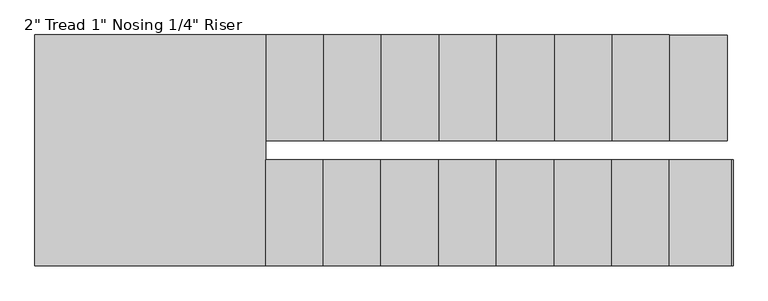
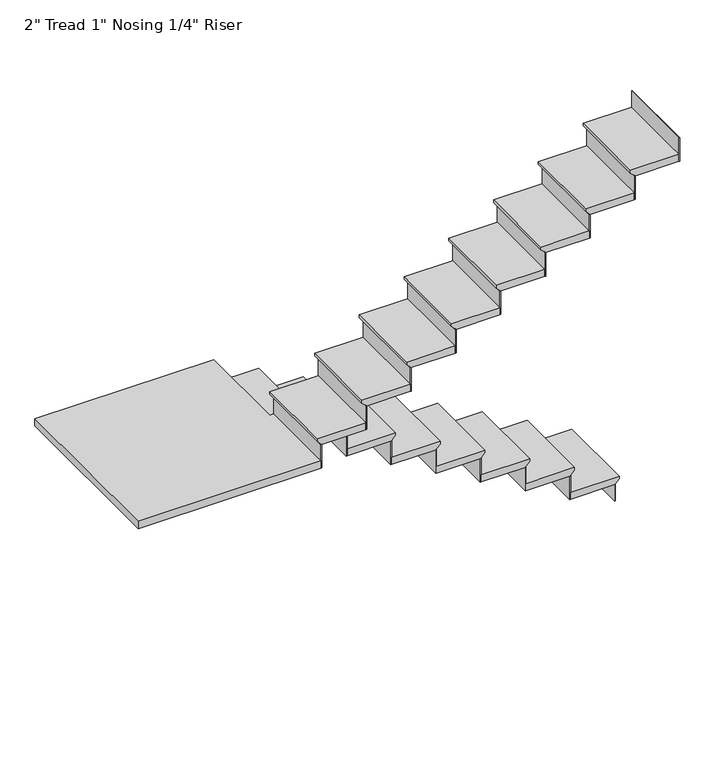
"""IFC4 building model written with IfcOpenShell, lengths in millimetres: stair flight geometry."""

from ifc_helpers import new_model, si_unit, origin, place, context, project, spatial, faceted_brep, source, transform, mapped, element, save


def stair_flight_b2054cc5(model_context):
    return source(origin(), model_context, "Body", "Brep", [
        faceted_brep([(-1805.9198569, -5306.3933037, 16152.2833333), (-1805.9198569, -5306.3933037, 16171.3333333), (-1805.9198569, -5865.1933037, 16171.3333333), (-1805.9198569, -5865.1933037, 16152.2833333), (-1831.3198569, -5306.3933037, 16126.8833333), (-1831.3198569, -5865.1933037, 16126.8833333), (-2136.1198569, -5306.3933037, 16171.3333333), (-2136.1198569, -5865.1933037, 16171.3333333), (-1831.3198569, -5865.1933037, 16120.5333333), (-2136.1198569, -5865.1933037, 16120.5333333), (-2136.1198569, -5306.3933037, 16120.5333333), (-1831.3198569, -5306.3933037, 16120.5333333)], [[[0, 1, 2, 3]], [[4, 0, 3, 5]], [[2, 1, 6, 7]], [[8, 9, 10, 11]], [[2, 7, 9, 8, 5, 3]], [[8, 11, 4, 5]], [[6, 1, 0, 4, 11, 10]], [[7, 6, 10, 9]]]),
        faceted_brep([(-1831.3198569, -5306.3933037, 16120.5333333), (-1831.3198569, -5306.3933037, 16002.0), (-1837.6698569, -5306.3933037, 16002.0), (-1837.6698569, -5306.3933037, 16120.5333333), (-1831.3198569, -5865.1933037, 16120.5333333), (-1837.6698569, -5865.1933037, 16120.5333333), (-1837.6698569, -5865.1933037, 16002.0), (-1831.3198569, -5865.1933037, 16002.0)], [[[0, 1, 2, 3]], [[4, 5, 6, 7]], [[1, 0, 4, 7]], [[2, 1, 7, 6]], [[3, 2, 6, 5]], [[0, 3, 5, 4]]]),
        faceted_brep([(-2136.1198569, -5306.3933037, 16289.8666667), (-2136.1198569, -5306.3933037, 16120.5333333), (-2142.4698569, -5306.3933037, 16120.5333333), (-2142.4698569, -5306.3933037, 16289.8666667), (-2136.1198569, -5865.1933037, 16289.8666667), (-2142.4698569, -5865.1933037, 16289.8666667), (-2142.4698569, -5865.1933037, 16120.5333333), (-2136.1198569, -5865.1933037, 16120.5333333)], [[[0, 1, 2, 3]], [[4, 5, 6, 7]], [[1, 0, 4, 7]], [[2, 1, 7, 6]], [[3, 2, 6, 5]], [[0, 3, 5, 4]]]),
        faceted_brep([(-2110.7198569, -5865.1933037, 16340.6666667), (-2110.7198569, -5306.3933037, 16340.6666667), (-2440.9198569, -5306.3933037, 16340.6666667), (-2440.9198569, -5865.1933037, 16340.6666667), (-2136.1198569, -5865.1933037, 16289.8666667), (-2440.9198569, -5865.1933037, 16289.8666667), (-2440.9198569, -5306.3933037, 16289.8666667), (-2136.1198569, -5306.3933037, 16289.8666667), (-2136.1198569, -5865.1933037, 16296.2166667), (-2110.7198569, -5865.1933037, 16321.6166667), (-2136.1198569, -5306.3933037, 16296.2166667), (-2110.7198569, -5306.3933037, 16321.6166667)], [[[0, 1, 2, 3]], [[4, 5, 6, 7]], [[0, 3, 5, 4, 8, 9]], [[4, 7, 10, 8]], [[2, 1, 11, 10, 7, 6]], [[3, 2, 6, 5]], [[11, 1, 0, 9]], [[10, 11, 9, 8]]]),
        faceted_brep([(-2440.9198569, -5306.3933037, 16459.2), (-2440.9198569, -5306.3933037, 16289.8666667), (-2447.2698569, -5306.3933037, 16289.8666667), (-2447.2698569, -5306.3933037, 16459.2), (-2440.9198569, -5865.1933037, 16459.2), (-2447.2698569, -5865.1933037, 16459.2), (-2447.2698569, -5865.1933037, 16289.8666667), (-2440.9198569, -5865.1933037, 16289.8666667)], [[[0, 1, 2, 3]], [[4, 5, 6, 7]], [[1, 0, 4, 7]], [[2, 1, 7, 6]], [[3, 2, 6, 5]], [[0, 3, 5, 4]]]),
        faceted_brep([(-2415.5198569, -5865.1933037, 16510.0), (-2415.5198569, -5306.3933037, 16510.0), (-2745.7198569, -5306.3933037, 16510.0), (-2745.7198569, -5865.1933037, 16510.0), (-2440.9198569, -5865.1933037, 16459.2), (-2745.7198569, -5865.1933037, 16459.2), (-2745.7198569, -5306.3933037, 16459.2), (-2440.9198569, -5306.3933037, 16459.2), (-2440.9198569, -5865.1933037, 16465.55), (-2415.5198569, -5865.1933037, 16490.95), (-2440.9198569, -5306.3933037, 16465.55), (-2415.5198569, -5306.3933037, 16490.95)], [[[0, 1, 2, 3]], [[4, 5, 6, 7]], [[0, 3, 5, 4, 8, 9]], [[4, 7, 10, 8]], [[2, 1, 11, 10, 7, 6]], [[3, 2, 6, 5]], [[11, 1, 0, 9]], [[10, 11, 9, 8]]]),
        faceted_brep([(-2745.7198569, -5306.3933037, 16628.5333333), (-2745.7198569, -5306.3933037, 16459.2), (-2752.0698569, -5306.3933037, 16459.2), (-2752.0698569, -5306.3933037, 16628.5333333), (-2745.7198569, -5865.1933037, 16628.5333333), (-2752.0698569, -5865.1933037, 16628.5333333), (-2752.0698569, -5865.1933037, 16459.2), (-2745.7198569, -5865.1933037, 16459.2)], [[[0, 1, 2, 3]], [[4, 5, 6, 7]], [[1, 0, 4, 7]], [[2, 1, 7, 6]], [[3, 2, 6, 5]], [[0, 3, 5, 4]]]),
        faceted_brep([(-2720.3198569, -5865.1933037, 16679.3333333), (-2720.3198569, -5306.3933037, 16679.3333333), (-3050.5198569, -5306.3933037, 16679.3333333), (-3050.5198569, -5865.1933037, 16679.3333333), (-2745.7198569, -5865.1933037, 16628.5333333), (-3050.5198569, -5865.1933037, 16628.5333333), (-3050.5198569, -5306.3933037, 16628.5333333), (-2745.7198569, -5306.3933037, 16628.5333333), (-2745.7198569, -5865.1933037, 16634.8833333), (-2720.3198569, -5865.1933037, 16660.2833333), (-2745.7198569, -5306.3933037, 16634.8833333), (-2720.3198569, -5306.3933037, 16660.2833333)], [[[0, 1, 2, 3]], [[4, 5, 6, 7]], [[0, 3, 5, 4, 8, 9]], [[4, 7, 10, 8]], [[2, 1, 11, 10, 7, 6]], [[3, 2, 6, 5]], [[11, 1, 0, 9]], [[10, 11, 9, 8]]]),
        faceted_brep([(-3050.5198569, -5306.3933037, 16797.8666667), (-3050.5198569, -5306.3933037, 16628.5333333), (-3056.8698569, -5306.3933037, 16628.5333333), (-3056.8698569, -5306.3933037, 16797.8666667), (-3050.5198569, -5865.1933037, 16797.8666667), (-3056.8698569, -5865.1933037, 16797.8666667), (-3056.8698569, -5865.1933037, 16628.5333333), (-3050.5198569, -5865.1933037, 16628.5333333)], [[[0, 1, 2, 3]], [[4, 5, 6, 7]], [[1, 0, 4, 7]], [[2, 1, 7, 6]], [[3, 2, 6, 5]], [[0, 3, 5, 4]]]),
        faceted_brep([(-3025.1198569, -5865.1933037, 16848.6666667), (-3025.1198569, -5306.3933037, 16848.6666667), (-3355.3198569, -5306.3933037, 16848.6666667), (-3355.3198569, -5865.1933037, 16848.6666667), (-3050.5198569, -5865.1933037, 16797.8666667), (-3355.3198569, -5865.1933037, 16797.8666667), (-3355.3198569, -5306.3933037, 16797.8666667), (-3050.5198569, -5306.3933037, 16797.8666667), (-3050.5198569, -5865.1933037, 16804.2166667), (-3025.1198569, -5865.1933037, 16829.6166667), (-3050.5198569, -5306.3933037, 16804.2166667), (-3025.1198569, -5306.3933037, 16829.6166667)], [[[0, 1, 2, 3]], [[4, 5, 6, 7]], [[0, 3, 5, 4, 8, 9]], [[4, 7, 10, 8]], [[2, 1, 11, 10, 7, 6]], [[3, 2, 6, 5]], [[11, 1, 0, 9]], [[10, 11, 9, 8]]]),
        faceted_brep([(-3355.3198569, -5306.3933037, 16967.2), (-3355.3198569, -5306.3933037, 16797.8666667), (-3361.6698569, -5306.3933037, 16797.8666667), (-3361.6698569, -5306.3933037, 16967.2), (-3355.3198569, -5865.1933037, 16967.2), (-3361.6698569, -5865.1933037, 16967.2), (-3361.6698569, -5865.1933037, 16797.8666667), (-3355.3198569, -5865.1933037, 16797.8666667)], [[[0, 1, 2, 3]], [[4, 5, 6, 7]], [[1, 0, 4, 7]], [[2, 1, 7, 6]], [[3, 2, 6, 5]], [[0, 3, 5, 4]]]),
        faceted_brep([(-3329.9198569, -5865.1933037, 17018.0), (-3329.9198569, -5306.3933037, 17018.0), (-3660.1198569, -5306.3933037, 17018.0), (-3660.1198569, -5865.1933037, 17018.0), (-3355.3198569, -5865.1933037, 16967.2), (-3660.1198569, -5865.1933037, 16967.2), (-3660.1198569, -5306.3933037, 16967.2), (-3355.3198569, -5306.3933037, 16967.2), (-3355.3198569, -5865.1933037, 16973.55), (-3329.9198569, -5865.1933037, 16998.95), (-3355.3198569, -5306.3933037, 16973.55), (-3329.9198569, -5306.3933037, 16998.95)], [[[0, 1, 2, 3]], [[4, 5, 6, 7]], [[0, 3, 5, 4, 8, 9]], [[4, 7, 10, 8]], [[2, 1, 11, 10, 7, 6]], [[3, 2, 6, 5]], [[11, 1, 0, 9]], [[10, 11, 9, 8]]]),
        faceted_brep([(-3660.1198569, -5306.3933037, 17136.5333333), (-3660.1198569, -5306.3933037, 16967.2), (-3666.4698569, -5306.3933037, 16967.2), (-3666.4698569, -5306.3933037, 17136.5333333), (-3660.1198569, -5865.1933037, 17136.5333333), (-3666.4698569, -5865.1933037, 17136.5333333), (-3666.4698569, -5865.1933037, 16967.2), (-3660.1198569, -5865.1933037, 16967.2)], [[[0, 1, 2, 3]], [[4, 5, 6, 7]], [[1, 0, 4, 7]], [[2, 1, 7, 6]], [[3, 2, 6, 5]], [[0, 3, 5, 4]]]),
        faceted_brep([(-3634.7198569, -5865.1933037, 17187.3333333), (-3634.7198569, -5306.3933037, 17187.3333333), (-3964.9198569, -5306.3933037, 17187.3333333), (-3964.9198569, -5865.1933037, 17187.3333333), (-3660.1198569, -5865.1933037, 17136.5333333), (-3964.9198569, -5865.1933037, 17136.5333333), (-3964.9198569, -5306.3933037, 17136.5333333), (-3660.1198569, -5306.3933037, 17136.5333333), (-3660.1198569, -5865.1933037, 17142.8833333), (-3634.7198569, -5865.1933037, 17168.2833333), (-3660.1198569, -5306.3933037, 17142.8833333), (-3634.7198569, -5306.3933037, 17168.2833333)], [[[0, 1, 2, 3]], [[4, 5, 6, 7]], [[0, 3, 5, 4, 8, 9]], [[4, 7, 10, 8]], [[2, 1, 11, 10, 7, 6]], [[3, 2, 6, 5]], [[11, 1, 0, 9]], [[10, 11, 9, 8]]]),
        faceted_brep([(-3964.9198569, -5306.3933037, 17305.8666667), (-3964.9198569, -5306.3933037, 17136.5333333), (-3971.2698569, -5306.3933037, 17136.5333333), (-3971.2698569, -5306.3933037, 17305.8666667), (-3964.9198569, -5865.1933037, 17305.8666667), (-3971.2698569, -5865.1933037, 17305.8666667), (-3971.2698569, -5865.1933037, 17136.5333333), (-3964.9198569, -5865.1933037, 17136.5333333)], [[[0, 1, 2, 3]], [[4, 5, 6, 7]], [[1, 0, 4, 7]], [[2, 1, 7, 6]], [[3, 2, 6, 5]], [[0, 3, 5, 4]]]),
        faceted_brep([(-3939.5198569, -5865.1933037, 17356.6666667), (-3939.5198569, -5306.3933037, 17356.6666667), (-4269.7198569, -5306.3933037, 17356.6666667), (-4269.7198569, -5865.1933037, 17356.6666667), (-3964.9198569, -5865.1933037, 17305.8666667), (-4269.7198569, -5865.1933037, 17305.8666667), (-4269.7198569, -5306.3933037, 17305.8666667), (-3964.9198569, -5306.3933037, 17305.8666667), (-3964.9198569, -5865.1933037, 17312.2166667), (-3939.5198569, -5865.1933037, 17337.6166667), (-3964.9198569, -5306.3933037, 17312.2166667), (-3939.5198569, -5306.3933037, 17337.6166667)], [[[0, 1, 2, 3]], [[4, 5, 6, 7]], [[0, 3, 5, 4, 8, 9]], [[4, 7, 10, 8]], [[2, 1, 11, 10, 7, 6]], [[3, 2, 6, 5]], [[11, 1, 0, 9]], [[10, 11, 9, 8]]]),
        faceted_brep([(-4269.7198569, -5306.3933037, 17475.2), (-4269.7198569, -5306.3933037, 17305.8666667), (-4276.0698569, -5306.3933037, 17305.8666667), (-4276.0698569, -5306.3933037, 17475.2), (-4269.7198569, -5865.1933037, 17475.2), (-4276.0698569, -5865.1933037, 17475.2), (-4276.0698569, -5865.1933037, 17305.8666667), (-4269.7198569, -5865.1933037, 17305.8666667)], [[[0, 1, 2, 3]], [[4, 5, 6, 7]], [[1, 0, 4, 7]], [[2, 1, 7, 6]], [[3, 2, 6, 5]], [[0, 3, 5, 4]]]),
        faceted_brep([(-4218.9198569, -5966.7933037, 17526.0), (-4244.3198569, -5966.7933037, 17526.0), (-4244.3198569, -5306.3933037, 17526.0), (-5463.5198569, -5306.3933037, 17526.0), (-5463.5198569, -6525.5933037, 17526.0), (-4218.9198569, -6525.5933037, 17526.0), (-4244.3198569, -5966.7933037, 17475.2), (-4218.9198569, -5966.7933037, 17475.2), (-4218.9198569, -6525.5933037, 17475.2), (-5463.5198569, -6525.5933037, 17475.2), (-5463.5198569, -5306.3933037, 17475.2), (-4269.7198569, -5306.3933037, 17475.2), (-4269.7198569, -5865.1933037, 17475.2), (-4244.3198569, -5865.1933037, 17475.2), (-4244.3198569, -5865.1933037, 17506.95), (-4244.3198569, -5306.3933037, 17506.95), (-4269.7198569, -5865.1933037, 17481.55), (-4269.7198569, -5306.3933037, 17481.55)], [[[0, 1, 2, 3, 4, 5]], [[6, 7, 8, 9, 10, 11, 12, 13]], [[1, 0, 7, 6]], [[2, 1, 6, 13, 14, 15]], [[13, 12, 16, 14]], [[12, 11, 17, 16]], [[3, 2, 15, 17, 11, 10]], [[4, 3, 10, 9]], [[5, 4, 9, 8]], [[0, 5, 8, 7]], [[17, 15, 14, 16]]]),
        faceted_brep([(-4218.9198569, -6525.5933037, 17644.5333333), (-4218.9198569, -6525.5933037, 17475.2), (-4212.5698569, -6525.5933037, 17475.2), (-4212.5698569, -6525.5933037, 17644.5333333), (-4218.9198569, -5966.7933037, 17644.5333333), (-4212.5698569, -5966.7933037, 17644.5333333), (-4212.5698569, -5966.7933037, 17475.2), (-4218.9198569, -5966.7933037, 17475.2)], [[[0, 1, 2, 3]], [[4, 5, 6, 7]], [[1, 0, 4, 7]], [[2, 1, 7, 6]], [[3, 2, 6, 5]], [[0, 3, 5, 4]]]),
        faceted_brep([(-4244.3198569, -5966.7933037, 17695.3333333), (-4244.3198569, -6525.5933037, 17695.3333333), (-3914.1198569, -6525.5933037, 17695.3333333), (-3914.1198569, -5966.7933037, 17695.3333333), (-4218.9198569, -5966.7933037, 17644.5333333), (-3914.1198569, -5966.7933037, 17644.5333333), (-3914.1198569, -6525.5933037, 17644.5333333), (-4218.9198569, -6525.5933037, 17644.5333333), (-4218.9198569, -5966.7933037, 17650.8833333), (-4244.3198569, -5966.7933037, 17676.2833333), (-4218.9198569, -6525.5933037, 17650.8833333), (-4244.3198569, -6525.5933037, 17676.2833333)], [[[0, 1, 2, 3]], [[4, 5, 6, 7]], [[0, 3, 5, 4, 8, 9]], [[4, 7, 10, 8]], [[2, 1, 11, 10, 7, 6]], [[3, 2, 6, 5]], [[11, 1, 0, 9]], [[10, 11, 9, 8]]]),
        faceted_brep([(-3914.1198569, -6525.5933037, 17813.8666667), (-3914.1198569, -6525.5933037, 17644.5333333), (-3907.7698569, -6525.5933037, 17644.5333333), (-3907.7698569, -6525.5933037, 17813.8666667), (-3914.1198569, -5966.7933037, 17813.8666667), (-3907.7698569, -5966.7933037, 17813.8666667), (-3907.7698569, -5966.7933037, 17644.5333333), (-3914.1198569, -5966.7933037, 17644.5333333)], [[[0, 1, 2, 3]], [[4, 5, 6, 7]], [[1, 0, 4, 7]], [[2, 1, 7, 6]], [[3, 2, 6, 5]], [[0, 3, 5, 4]]]),
        faceted_brep([(-3939.5198569, -5966.7933037, 17864.6666667), (-3939.5198569, -6525.5933037, 17864.6666667), (-3609.3198569, -6525.5933037, 17864.6666667), (-3609.3198569, -5966.7933037, 17864.6666667), (-3914.1198569, -5966.7933037, 17813.8666667), (-3609.3198569, -5966.7933037, 17813.8666667), (-3609.3198569, -6525.5933037, 17813.8666667), (-3914.1198569, -6525.5933037, 17813.8666667), (-3914.1198569, -5966.7933037, 17820.2166667), (-3939.5198569, -5966.7933037, 17845.6166667), (-3914.1198569, -6525.5933037, 17820.2166667), (-3939.5198569, -6525.5933037, 17845.6166667)], [[[0, 1, 2, 3]], [[4, 5, 6, 7]], [[0, 3, 5, 4, 8, 9]], [[4, 7, 10, 8]], [[2, 1, 11, 10, 7, 6]], [[3, 2, 6, 5]], [[11, 1, 0, 9]], [[10, 11, 9, 8]]]),
        faceted_brep([(-3609.3198569, -6525.5933037, 17983.2), (-3609.3198569, -6525.5933037, 17813.8666667), (-3602.9698569, -6525.5933037, 17813.8666667), (-3602.9698569, -6525.5933037, 17983.2), (-3609.3198569, -5966.7933037, 17983.2), (-3602.9698569, -5966.7933037, 17983.2), (-3602.9698569, -5966.7933037, 17813.8666667), (-3609.3198569, -5966.7933037, 17813.8666667)], [[[0, 1, 2, 3]], [[4, 5, 6, 7]], [[1, 0, 4, 7]], [[2, 1, 7, 6]], [[3, 2, 6, 5]], [[0, 3, 5, 4]]]),
        faceted_brep([(-3634.7198569, -5966.7933037, 18034.0), (-3634.7198569, -6525.5933037, 18034.0), (-3304.5198569, -6525.5933037, 18034.0), (-3304.5198569, -5966.7933037, 18034.0), (-3609.3198569, -5966.7933037, 17983.2), (-3304.5198569, -5966.7933037, 17983.2), (-3304.5198569, -6525.5933037, 17983.2), (-3609.3198569, -6525.5933037, 17983.2), (-3609.3198569, -5966.7933037, 17989.55), (-3634.7198569, -5966.7933037, 18014.95), (-3609.3198569, -6525.5933037, 17989.55), (-3634.7198569, -6525.5933037, 18014.95)], [[[0, 1, 2, 3]], [[4, 5, 6, 7]], [[0, 3, 5, 4, 8, 9]], [[4, 7, 10, 8]], [[2, 1, 11, 10, 7, 6]], [[3, 2, 6, 5]], [[11, 1, 0, 9]], [[10, 11, 9, 8]]]),
        faceted_brep([(-3304.5198569, -6525.5933037, 18152.5333333), (-3304.5198569, -6525.5933037, 17983.2), (-3298.1698569, -6525.5933037, 17983.2), (-3298.1698569, -6525.5933037, 18152.5333333), (-3304.5198569, -5966.7933037, 18152.5333333), (-3298.1698569, -5966.7933037, 18152.5333333), (-3298.1698569, -5966.7933037, 17983.2), (-3304.5198569, -5966.7933037, 17983.2)], [[[0, 1, 2, 3]], [[4, 5, 6, 7]], [[1, 0, 4, 7]], [[2, 1, 7, 6]], [[3, 2, 6, 5]], [[0, 3, 5, 4]]]),
        faceted_brep([(-3329.9198569, -5966.7933037, 18203.3333333), (-3329.9198569, -6525.5933037, 18203.3333333), (-2999.7198569, -6525.5933037, 18203.3333333), (-2999.7198569, -5966.7933037, 18203.3333333), (-3304.5198569, -5966.7933037, 18152.5333333), (-2999.7198569, -5966.7933037, 18152.5333333), (-2999.7198569, -6525.5933037, 18152.5333333), (-3304.5198569, -6525.5933037, 18152.5333333), (-3304.5198569, -5966.7933037, 18158.8833333), (-3329.9198569, -5966.7933037, 18184.2833333), (-3304.5198569, -6525.5933037, 18158.8833333), (-3329.9198569, -6525.5933037, 18184.2833333)], [[[0, 1, 2, 3]], [[4, 5, 6, 7]], [[0, 3, 5, 4, 8, 9]], [[4, 7, 10, 8]], [[2, 1, 11, 10, 7, 6]], [[3, 2, 6, 5]], [[11, 1, 0, 9]], [[10, 11, 9, 8]]]),
        faceted_brep([(-2999.7198569, -6525.5933037, 18321.8666667), (-2999.7198569, -6525.5933037, 18152.5333333), (-2993.3698569, -6525.5933037, 18152.5333333), (-2993.3698569, -6525.5933037, 18321.8666667), (-2999.7198569, -5966.7933037, 18321.8666667), (-2993.3698569, -5966.7933037, 18321.8666667), (-2993.3698569, -5966.7933037, 18152.5333333), (-2999.7198569, -5966.7933037, 18152.5333333)], [[[0, 1, 2, 3]], [[4, 5, 6, 7]], [[1, 0, 4, 7]], [[2, 1, 7, 6]], [[3, 2, 6, 5]], [[0, 3, 5, 4]]]),
        faceted_brep([(-3025.1198569, -5966.7933037, 18372.6666667), (-3025.1198569, -6525.5933037, 18372.6666667), (-2694.9198569, -6525.5933037, 18372.6666667), (-2694.9198569, -5966.7933037, 18372.6666667), (-2999.7198569, -5966.7933037, 18321.8666667), (-2694.9198569, -5966.7933037, 18321.8666667), (-2694.9198569, -6525.5933037, 18321.8666667), (-2999.7198569, -6525.5933037, 18321.8666667), (-2999.7198569, -5966.7933037, 18328.2166667), (-3025.1198569, -5966.7933037, 18353.6166667), (-2999.7198569, -6525.5933037, 18328.2166667), (-3025.1198569, -6525.5933037, 18353.6166667)], [[[0, 1, 2, 3]], [[4, 5, 6, 7]], [[0, 3, 5, 4, 8, 9]], [[4, 7, 10, 8]], [[2, 1, 11, 10, 7, 6]], [[3, 2, 6, 5]], [[11, 1, 0, 9]], [[10, 11, 9, 8]]]),
        faceted_brep([(-2694.9198569, -6525.5933037, 18491.2), (-2694.9198569, -6525.5933037, 18321.8666667), (-2688.5698569, -6525.5933037, 18321.8666667), (-2688.5698569, -6525.5933037, 18491.2), (-2694.9198569, -5966.7933037, 18491.2), (-2688.5698569, -5966.7933037, 18491.2), (-2688.5698569, -5966.7933037, 18321.8666667), (-2694.9198569, -5966.7933037, 18321.8666667)], [[[0, 1, 2, 3]], [[4, 5, 6, 7]], [[1, 0, 4, 7]], [[2, 1, 7, 6]], [[3, 2, 6, 5]], [[0, 3, 5, 4]]]),
        faceted_brep([(-2720.3198569, -5966.7933037, 18542.0), (-2720.3198569, -6525.5933037, 18542.0), (-2390.1198569, -6525.5933037, 18542.0), (-2390.1198569, -5966.7933037, 18542.0), (-2694.9198569, -5966.7933037, 18491.2), (-2390.1198569, -5966.7933037, 18491.2), (-2390.1198569, -6525.5933037, 18491.2), (-2694.9198569, -6525.5933037, 18491.2), (-2694.9198569, -5966.7933037, 18497.55), (-2720.3198569, -5966.7933037, 18522.95), (-2694.9198569, -6525.5933037, 18497.55), (-2720.3198569, -6525.5933037, 18522.95)], [[[0, 1, 2, 3]], [[4, 5, 6, 7]], [[0, 3, 5, 4, 8, 9]], [[4, 7, 10, 8]], [[2, 1, 11, 10, 7, 6]], [[3, 2, 6, 5]], [[11, 1, 0, 9]], [[10, 11, 9, 8]]]),
        faceted_brep([(-2390.1198569, -6525.5933037, 18660.5333333), (-2390.1198569, -6525.5933037, 18491.2), (-2383.7698569, -6525.5933037, 18491.2), (-2383.7698569, -6525.5933037, 18660.5333333), (-2390.1198569, -5966.7933037, 18660.5333333), (-2383.7698569, -5966.7933037, 18660.5333333), (-2383.7698569, -5966.7933037, 18491.2), (-2390.1198569, -5966.7933037, 18491.2)], [[[0, 1, 2, 3]], [[4, 5, 6, 7]], [[1, 0, 4, 7]], [[2, 1, 7, 6]], [[3, 2, 6, 5]], [[0, 3, 5, 4]]]),
        faceted_brep([(-2415.5198569, -5966.7933037, 18711.3333333), (-2415.5198569, -6525.5933037, 18711.3333333), (-2085.3198569, -6525.5933037, 18711.3333333), (-2085.3198569, -5966.7933037, 18711.3333333), (-2390.1198569, -5966.7933037, 18660.5333333), (-2085.3198569, -5966.7933037, 18660.5333333), (-2085.3198569, -6525.5933037, 18660.5333333), (-2390.1198569, -6525.5933037, 18660.5333333), (-2390.1198569, -5966.7933037, 18666.8833333), (-2415.5198569, -5966.7933037, 18692.2833333), (-2390.1198569, -6525.5933037, 18666.8833333), (-2415.5198569, -6525.5933037, 18692.2833333)], [[[0, 1, 2, 3]], [[4, 5, 6, 7]], [[0, 3, 5, 4, 8, 9]], [[4, 7, 10, 8]], [[2, 1, 11, 10, 7, 6]], [[3, 2, 6, 5]], [[11, 1, 0, 9]], [[10, 11, 9, 8]]]),
        faceted_brep([(-2085.3198569, -6525.5933037, 18829.8666667), (-2085.3198569, -6525.5933037, 18660.5333333), (-2078.9698569, -6525.5933037, 18660.5333333), (-2078.9698569, -6525.5933037, 18829.8666667), (-2085.3198569, -5966.7933037, 18829.8666667), (-2078.9698569, -5966.7933037, 18829.8666667), (-2078.9698569, -5966.7933037, 18660.5333333), (-2085.3198569, -5966.7933037, 18660.5333333)], [[[0, 1, 2, 3]], [[4, 5, 6, 7]], [[1, 0, 4, 7]], [[2, 1, 7, 6]], [[3, 2, 6, 5]], [[0, 3, 5, 4]]]),
        faceted_brep([(-1780.5198569, -6525.5933037, 18999.2), (-1780.5198569, -6525.5933037, 18829.8666667), (-1774.1698569, -6525.5933037, 18829.8666667), (-1774.1698569, -6525.5933037, 18999.2), (-1780.5198569, -5966.7933037, 18999.2), (-1774.1698569, -5966.7933037, 18999.2), (-1774.1698569, -5966.7933037, 18829.8666667), (-1780.5198569, -5966.7933037, 18829.8666667)], [[[0, 1, 2, 3]], [[4, 5, 6, 7]], [[1, 0, 4, 7]], [[2, 1, 7, 6]], [[3, 2, 6, 5]], [[0, 3, 5, 4]]]),
        faceted_brep([(-2110.7198569, -5966.7933037, 18880.6666667), (-2110.7198569, -6525.5933037, 18880.6666667), (-1780.5198569, -6525.5933037, 18880.6666667), (-1780.5198569, -5966.7933037, 18880.6666667), (-2085.3198569, -5966.7933037, 18829.8666667), (-1780.5198569, -5966.7933037, 18829.8666667), (-1780.5198569, -6525.5933037, 18829.8666667), (-2085.3198569, -6525.5933037, 18829.8666667), (-2085.3198569, -5966.7933037, 18836.2166667), (-2110.7198569, -5966.7933037, 18861.6166667), (-2085.3198569, -6525.5933037, 18836.2166667), (-2110.7198569, -6525.5933037, 18861.6166667)], [[[0, 1, 2, 3]], [[4, 5, 6, 7]], [[0, 3, 5, 4, 8, 9]], [[4, 7, 10, 8]], [[2, 1, 11, 10, 7, 6]], [[3, 2, 6, 5]], [[11, 1, 0, 9]], [[10, 11, 9, 8]]]),
    ])


if __name__ == "__main__":
    model = new_model("IFC4")
    model_context = context("Model", 3, world=origin())
    ifc_project = project(units=[si_unit("LENGTHUNIT", "METRE", prefix="MILLI")], contexts=[model_context])
    site = spatial("IfcSite", under=ifc_project)
    building = spatial("IfcBuilding", under=site)
    placement = place(None, origin())
    stair_flight_shape = stair_flight_b2054cc5(model_context)
    element("IfcStairFlight", 1, ObjectType="2\" Tread 1\" Nosing 1/4\" Riser", at=placement, inside=building, context=model_context, shape_type="MappedRepresentation", body=[
        mapped(stair_flight_shape, transform((0.0, 0.0, 0.0), x_axis=(1.0, 0.0, 0.0), y_axis=(0.0, 1.0, 0.0), z_axis=(0.0, 0.0, 1.0))),
    ])
    save(model, "model.ifc")
